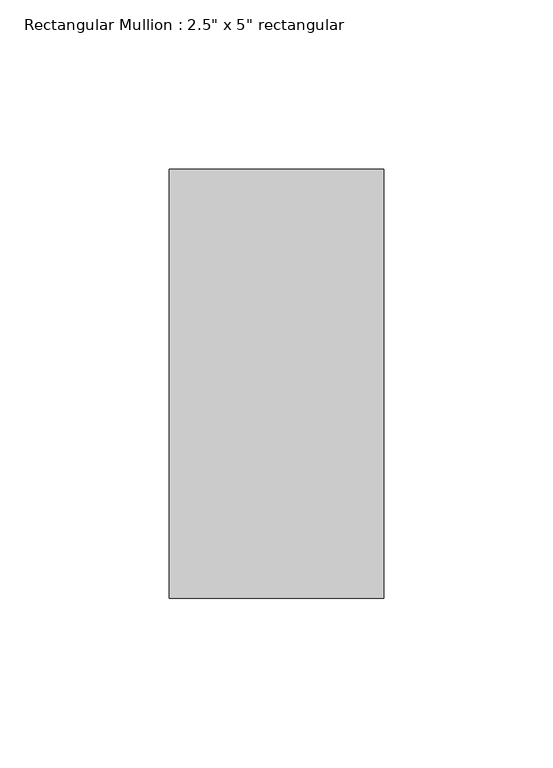
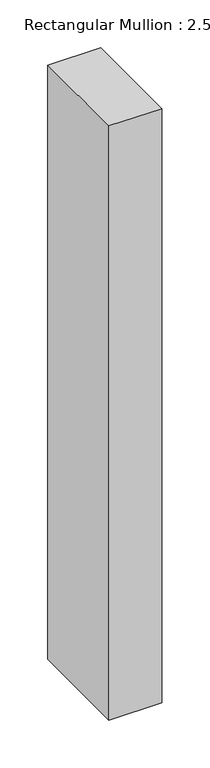
"""IFC4 building model written with IfcOpenShell, lengths in millimetres: member geometry."""

from ifc_helpers import new_model, si_unit, frame, origin, place, context, project, spatial, polyline, outline, extrude, source, transform, mapped, element, save


def member_a3a7b6e3(model_context):
    return source(origin(), model_context, "Body", "SweptSolid", [
        extrude(outline(polyline([(0.0, 63.5), (0.0, -63.5), (-63.5, -63.5), (-63.5, 63.5), (0.0, 63.5)])), frame((0.0, 0.0, -755.65), z_axis=(0.0, 0.0, 1.0), x_axis=(1.0, 0.0, 0.0)), (0.0, 0.0, 1.0), 755.65),
    ])


if __name__ == "__main__":
    model = new_model("IFC4")
    model_context = context("Model", 3, world=origin())
    ifc_project = project(units=[si_unit("LENGTHUNIT", "METRE", prefix="MILLI")], contexts=[model_context])
    site = spatial("IfcSite", under=ifc_project)
    building = spatial("IfcBuilding", under=site)
    placement = place(None, origin())
    member_shape = member_a3a7b6e3(model_context)
    element("IfcMember", 1, ObjectType="Rectangular Mullion : 2.5\" x 5\" rectangular", at=placement, inside=building, context=model_context, shape_type="MappedRepresentation", body=[
        mapped(member_shape, transform((0.0, 0.0, 0.0), x_axis=(1.0, 0.0, 0.0), y_axis=(0.0, 1.0, 0.0), z_axis=(0.0, 0.0, 1.0))),
    ])
    save(model, "model.ifc")

# Revit data of these elements
# Type "Rectangular Mullion : 2.5\" x 5\" rectangular"
#   built-in parameter 1007304 = 0.416667 (stored number, unit not read)
#   built-in parameter 1007301 = 0.104167 (stored number, unit not read)
#   built-in parameter 1007300 = 0.104167 (stored number, unit not read)
